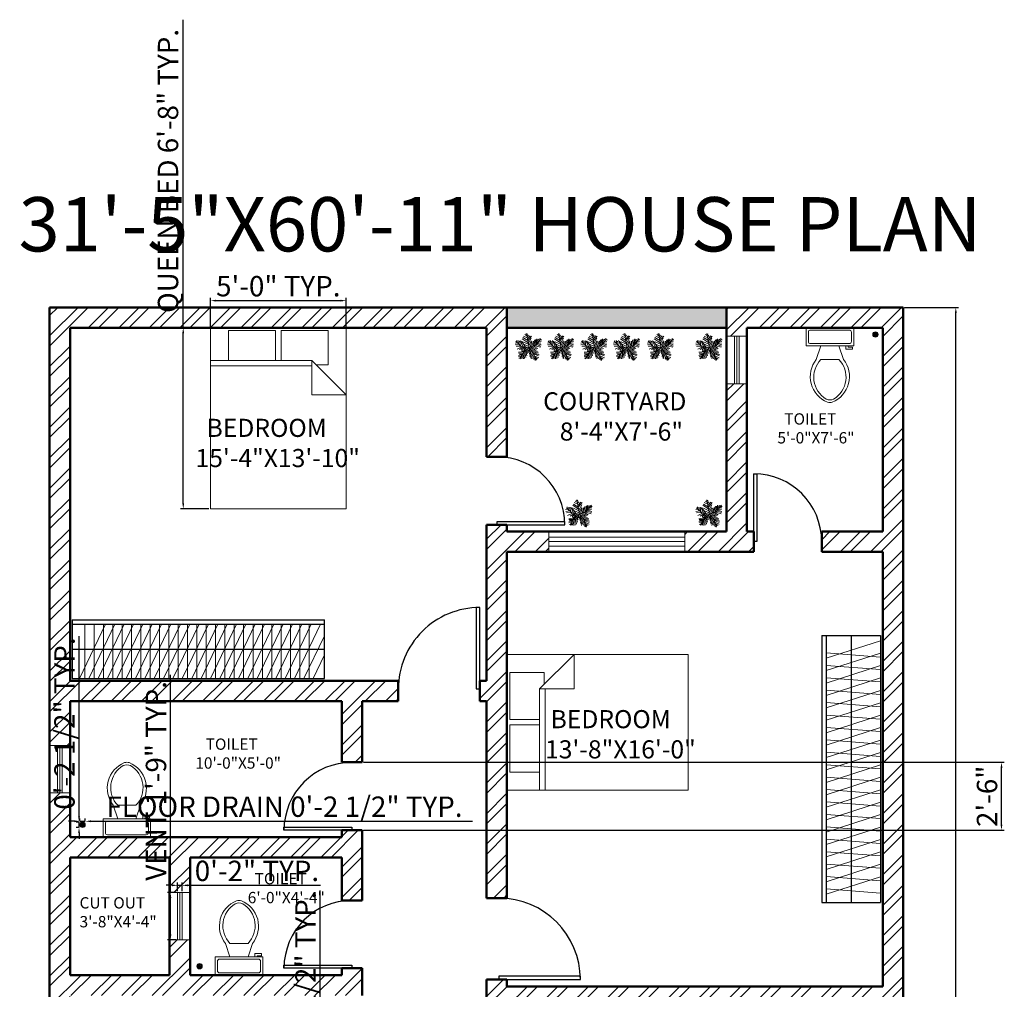
# Model space of a CAD drawing. Units: inches. Extents: x 764 to 1199, y 2696 to 3678.
# Tile 3 of 3: x 764 to 1199, y 3250 to 3678. Entities that reach past the tile are written whole.
import ezdxf

# ---------------------------------------------------------------- set-up
doc = ezdxf.new("R2010")
doc.units = ezdxf.units.IN
for name, color, linetype, lineweight in [('A-ANNO-DIMS', 2, 'Continuous', 18), ('A-ANNO-TITL', 7, 'Continuous', 35), ('A-AREA-IDEN', 7, 'Continuous', 18), ('A-DOOR', 4, 'Continuous', 25), ('A-FLOR-FIXT', 8, 'Continuous', 20), ('A-FURN', 8, 'Continuous', 18), ('A-GLAZ', 244, 'Continuous', 20), ('A-MILL', 8, 'Continuous', 25), ('A-MILL-PATT', 8, 'Continuous', 13), ('A-WALL', 7, 'Continuous', 50), ('A-WALL-PATT', 252, 'Continuous', 13), ('L-PLNT', 3, 'Continuous', 13), ('P-FLOR-DRAN', 8, 'Continuous', 18)]:
    doc.layers.add(name, color=color, linetype=linetype, lineweight=lineweight)
doc.styles.get("Standard").update_dxf_attribs({"font": 'arial.ttf'})
doc.dimstyles.new('ISO-25', dxfattribs={"dimtxt": 9, "dimasz": 2.5, "dimexe": 1.25, "dimexo": 0.625, "dimtad": 1, "dimlunit": 3, "dimtxsty": 'Standard', "dimcen": 2.5, "dimadec": 0, "dimazin": 0, "dimtfac": 1, "dimtmove": 0, "dimatfit": 3, "dimfxl": 1, "dimarcsym": 0})

# ---------------------------------------------------------------- blocks, each defined once
blk = doc.blocks.new('*U2')
for p, q in [((0, 0), (0, -6)), ((40, 0), (40, -6))]:
    blk.add_line(p, q)
blk.add_lwpolyline([(0, 0), (0, 40), (1.75, 40), (1.75, 0)], close=True)
blk.add_arc((0, 0), 40, 0, 90)
blk = doc.blocks.new('*U3')
for p, q in [((0, 0), (0, 6)), ((40, 0), (40, 6))]:
    blk.add_line(p, q)
blk.add_lwpolyline([(0, 0), (0, -40), (1.75, -40), (1.75, 0)], close=True)
blk.add_arc((0, 0), 40, 270, 0)
blk = doc.blocks.new('*U4')
for p, q in [((0, 0), (0, -6)), ((40, 0), (40, -6))]:
    blk.add_line(p, q)
blk.add_lwpolyline([(0, 0), (0, 40), (1.75, 40), (1.75, 0)], close=True)
blk.add_arc((0, 0), 40, 0, 90)
blk = doc.blocks.new('Bed - Queen')
for p, q in [((0, -80.00003), (0, 0)), ((0, 0), (59.99999, 0)), ((59.99999, 0), (59.99999, -80.00003)), ((7.99999, -1.2), (28.79998, -1.2)), ((7.99999, -14.4), (7.99999, -1.2)), ((28.79998, -1.2), (28.79998, -14.4)), ((31.19999, -1.2), (51.99999, -1.2)), ((31.19999, -14.4), (31.19999, -1.2)), ((51.99999, -1.2), (51.99999, -16.4)), ((0, -14.4), (44.8, -14.4)), ((44.8, -16.8), (0, -16.8)), ((59.99999, -29.6), (44.8, -14.4)), ((44.8, -14.4), (44.8, -29.6)), ((51.99999, -16.4), (46.79936, -16.4)), ((44.8, -29.6), (59.99999, -29.6)), ((59.99999, -80.00003), (0, -80.00003))]:
    blk.add_line(p, q)
blk = doc.blocks.new('*U9')
for p, q in [((9.5, -6), (9.5, -2)), ((-10, -8.5), (-8, -8.5)), ((-10, -9.5), (-10, -8.5)), ((-8, -8.5), (-8, -8)), ((-7, -8), (-7, -9.5)), ((-4, -8), (-6, -14)), ((4, -8), (6, -14)), ((-7, -9.5), (-10, -9.5)), ((4, -14), (-4, -14))]:
    blk.add_line(p, q)
blk.add_lwpolyline([(10.5, -8), (10.5, 0), (-10.5, 0), (-10.5, -8)], close=True)
for points in [[(-9.5, -2), (-9.5, -6)], [(8.5, -1), (-8.5, -1)], [(-8.5, -7), (8.5, -7)]]:
    blk.add_lwpolyline(points)
for centre, radius, start, end in [((-8.62, -1.88), 0.884, 81.8699, 188.1301), ((8.62, -1.88), 0.884, 351.8699, 98.1301), ((-8.62, -6.12), 0.884, 171.8699, 278.1301), ((8.62, -6.12), 0.884, 261.8699, 8.1301), ((3.52, -21.58), 12.17, 141.4691, 247.9714), ((4.2, -21.82), 11.33, 136.3677, 238.9468), ((-3.52, -21.58), 12.17, 292.0284, 38.5307), ((-4.2, -21.82), 11.33, 301.053, 43.6321), ((0, -27.88), 4, 245.7318, 294.2682), ((0, -29), 4, 254.8605, 285.1395)]:
    blk.add_arc(centre, radius, start, end)
blk = doc.blocks.new('*U13')
for p, q in [((-5.114, 28.097), (-24.676, 40.636)), ((-7.288, 39.707), (-21.778, 46.673)), ((-8.737, 47.138), (-17.069, 52.711)), ((-10.186, 53.64), (-13.084, 55.962)), ((0, 0), (-10.5, 57)), ((-9.099, 51.782), (-6.563, 55.962)), ((-7.65, 43.423), (-2.578, 49.46)), ((-5.839, 35.992), (4.667, 48.067)), ((-5.114, 27.632), (10.463, 46.673)), ((-47.498, 19.737), (-55.83, 18.344)), ((-40.615, 13.7), (-55.105, 10.913)), ((-31.5, 4.5), (-52.5, 25.5)), ((-33.37, 6.269), (-52.207, 5.34)), ((-48.585, 21.131), (-49.309, 29.026)), ((-28.299, 3.483), (-47.86, -5.805)), ((-43.513, 28.561), (-42.427, 15.558)), ((-38.442, 26.239), (-34.819, 7.663)), ((-21.416, 3.018), (-38.079, -8.128)), ((-35.544, 28.097), (-24.314, 3.947)), ((0, 0), (-31.5, 4.5)), ((-14.533, 2.09), (-30.834, 25.31)), ((-15.982, 2.09), (-30.11, -9.521)), ((-3.665, 19.273), (-27.574, 35.527)), ((-24.314, 23.917), (-2.941, 13.7)), ((0, 0), (-22.5, -19.5)), ((-6.563, 1.161), (-21.416, -8.128)), ((-20.691, 13.7), (-1.129, 4.876)), ((-2.941, 16.486), (8.652, 37.85)), ((-1.129, 6.734), (9.014, 26.704)), ((0, 0), (27, 9)), ((0, 0), (18, -22.5)), ((3.942, 1.625), (11.187, 24.381)), ((6.478, 1.625), (26.04, -8.592)), ((10.101, 3.483), (17.708, 26.239)), ((11.187, 3.483), (30.749, -5.805)), ((16.259, 5.805), (23.142, 31.348)), ((18.07, 5.805), (35.096, -3.483)), ((22.055, 7.198), (27.489, 32.277)), ((24.229, 7.663), (46.688, 1.625)), ((27, 9), (48, 36)), ((27.127, 9.056), (31.112, 35.992)), ((29.662, 12.307), (48.137, 6.269)), ((31.836, 30.883), (32.561, 16.486)), ((33.285, 16.486), (48.862, 10.913)), ((35.096, 32.741), (37.27, 22.524)), ((36.183, 19.737), (48.137, 17.88)), ((38.719, 34.134), (41.979, 28.561)), ((40.53, 25.775), (48.862, 24.846)), ((43.791, 29.954), (51.036, 30.883)), ((44.153, 36.456), (45.239, 32.741)), ((-17.431, -15.094), (-42.789, -18.809)), ((-28.299, -29.026), (-42.789, -31.348)), ((-24.314, -21.596), (-42.427, -22.06)), ((-30.834, -34.135), (-42.427, -35.528)), ((-26.849, -26.24), (-40.253, -25.775)), ((-22.5, -19.5), (-37.5, -45)), ((-32.646, -36.921), (-31.921, -44.352)), ((-15.257, -12.772), (-30.11, -12.772)), ((-29.023, -30.884), (-27.936, -43.887)), ((-25.038, -23.918), (-22.865, -45.281)), ((-20.691, -18.345), (-17.793, -44.352)), ((-6.563, -5.805), (-19.967, -9.985)), ((-17.069, -15.094), (-12.721, -40.172)), ((-13.446, -11.378), (-8.737, -32.741)), ((-9.461, -8.592), (-6.201, -23.453)), ((-4.752, -3.483), (-3.665, -14.629)), ((2.493, -3.019), (-1.491, -20.202)), ((1.769, -2.555), (24.229, -9.521)), ((5.029, -6.27), (2.131, -25.775)), ((9.014, -11.378), (3.58, -35.992)), ((14.085, -16.951), (6.478, -40.172)), ((7.565, -9.056), (32.198, -14.629)), ((18.07, -22.524), (8.289, -45.745)), ((12.274, -15.094), (36.907, -18.809)), ((20.244, -30.419), (15.897, -44.816)), ((16.259, -19.738), (36.183, -22.989)), ((18, -22.5), (27, -52.5)), ((18.433, -22.524), (40.53, -29.026)), ((19.157, -25.311), (38.719, -33.206)), ((22.78, -37.85), (19.519, -48.532)), ((21.331, -32.741), (39.081, -40.636)), ((22.78, -38.314), (34.372, -44.816)), ((-34.457, -39.708), (-40.978, -42.494)), ((24.591, -45.745), (23.142, -50.854)), ((24.591, -43.423), (30.749, -47.603)), ((26.764, -49.925), (28.213, -50.854))]:
    blk.add_line(p, q)
blk = doc.blocks.new('*D15')
at = {"layer": 'A-ANNO-DIMS', "color": 0, "lineweight": -2, "transparency": 16777216}
for p, q in [((1154.86, 3551.25), (1178.72, 3551.25)), ((1177.47, 2822.75), (1177.47, 3548.75)), ((1154.86, 2820.25), (1178.72, 2820.25))]:
    blk.add_line(p, q, dxfattribs=at)
at = {"layer": 'A-ANNO-DIMS', "color": 0, "transparency": 16777216}
for points in [[(1177.05, 3548.75), (1177.89, 3548.75), (1177.47, 3551.25)], [(1177.05, 2822.75), (1177.89, 2822.75), (1177.47, 2820.25)]]:
    blk.add_solid(points, dxfattribs=at)
at = {"layer": 'Defpoints', "color": 0, "transparency": 16777216}
for p in [(1154.24, 3551.25), (1177.47, 3551.25), (1154.24, 2820.25)]:
    blk.add_point(p, dxfattribs=at)
at = {"layer": 'A-ANNO-DIMS', "color": 0, "transparency": 16777216, "insert": (1172.25, 3185.75), "char_height": 9, "attachment_point": 5, "rotation": 90}
blk.add_mtext('60\'-11"', dxfattribs=at)
blk = doc.blocks.new('WIN-GLAZING-60IN')
for p, q in [((0, 4), (60, 4)), ((0, 2), (60, 2)), ((0, 0), (60, 0))]:
    blk.add_line(p, q)
blk = doc.blocks.new('VENT-GLAZING-21IN')
for p, q in [((0, 0), (0, 21)), ((1, 0), (1, 21)), ((2, 0), (2, 21))]:
    blk.add_line(p, q)
blk = doc.blocks.new('FLOOR-DRAIN-ROUND')
for p, q in [((0, 1.19), (2.38, 1.19)), ((2.06, 0.38), (0.32, 2)), ((0.42, 0.28), (1.96, 2.1)), ((1.19, 2.38), (1.19, 0))]:
    blk.add_line(p, q)
for radius in [1.19, 0.891]:
    blk.add_circle((1.19, 1.19), radius)
blk = doc.blocks.new('*D22')
at = {"layer": 'A-ANNO-DIMS', "color": 0, "lineweight": -2, "transparency": 16777216}
for p, q in [((830.59, 3292.75), (830.59, 3388.85)), ((833.11, 3292.75), (829.34, 3292.75)), ((830.59, 3274.25), (830.59, 3290.25)), ((833.11, 3271.75), (829.34, 3271.75))]:
    blk.add_line(p, q, dxfattribs=at)
at = {"layer": 'A-ANNO-DIMS', "color": 0, "transparency": 16777216}
for points in [[(830.17, 3290.25), (831, 3290.25), (830.59, 3292.75)], [(830.17, 3274.25), (831, 3274.25), (830.59, 3271.75)]]:
    blk.add_solid(points, dxfattribs=at)
at = {"layer": 'Defpoints', "color": 0, "transparency": 16777216}
for p in [(830.59, 3292.75), (833.74, 3292.75), (833.74, 3271.75)]:
    blk.add_point(p, dxfattribs=at)
at = {"layer": 'A-ANNO-DIMS', "color": 0, "transparency": 16777216, "insert": (825.37, 3342.05), "char_height": 9, "attachment_point": 5, "rotation": 90}
blk.add_mtext('VENT 1\'-9" TYP.', dxfattribs=at)
blk = doc.blocks.new('*D23')
at = {"layer": 'A-ANNO-DIMS', "color": 0, "lineweight": -2, "transparency": 16777216}
for p, q in [((833.74, 3293.38), (833.74, 3297.15)), ((835.74, 3293.38), (835.74, 3297.15)), ((831.24, 3295.9), (828.74, 3295.9)), ((833.74, 3295.9), (835.74, 3295.9)), ((838.24, 3295.9), (896.85, 3295.9))]:
    blk.add_line(p, q, dxfattribs=at)
at = {"layer": 'A-ANNO-DIMS', "color": 0, "transparency": 16777216}
for points in [[(831.24, 3296.32), (831.24, 3295.48), (833.74, 3295.9)], [(838.24, 3296.32), (838.24, 3295.48), (835.74, 3295.9)]]:
    blk.add_solid(points, dxfattribs=at)
at = {"layer": 'Defpoints', "color": 0, "transparency": 16777216}
for p in [(833.74, 3292.75), (835.74, 3295.9), (835.74, 3292.75)]:
    blk.add_point(p, dxfattribs=at)
at = {"layer": 'A-ANNO-DIMS', "color": 0, "transparency": 16777216, "insert": (868.79, 3301.12), "char_height": 9, "attachment_point": 5}
blk.add_mtext('0\'-2" TYP.', dxfattribs=at)
blk = doc.blocks.new('*D26')
at = {"layer": 'A-ANNO-DIMS', "color": 0, "lineweight": -2, "transparency": 16777216}
for p, q in [((788.08, 3324.2), (785.58, 3324.2)), ((790.58, 3324.47), (790.58, 3325.45)), ((790.58, 3324.2), (792.96, 3324.2)), ((792.96, 3324.47), (792.96, 3325.45)), ((795.46, 3324.2), (963.95, 3324.2))]:
    blk.add_line(p, q, dxfattribs=at)
at = {"layer": 'A-ANNO-DIMS', "color": 0, "transparency": 16777216}
for points in [[(788.08, 3324.62), (788.08, 3323.78), (790.58, 3324.2)], [(795.46, 3324.62), (795.46, 3323.78), (792.96, 3324.2)]]:
    blk.add_solid(points, dxfattribs=at)
at = {"layer": 'Defpoints', "color": 0, "transparency": 16777216}
for p in [(790.58, 3323.84), (792.96, 3324.2), (792.96, 3323.84)]:
    blk.add_point(p, dxfattribs=at)
at = {"layer": 'A-ANNO-DIMS', "color": 0, "transparency": 16777216, "insert": (880.96, 3329.48), "char_height": 9, "attachment_point": 5}
blk.add_mtext('FLOOR DRAIN 0\'-2 1/2" TYP.', dxfattribs=at)
blk = doc.blocks.new('*D27')
at = {"layer": 'A-ANNO-DIMS', "color": 0, "lineweight": -2, "transparency": 16777216}
for p, q in [((790.22, 3326.34), (790.22, 3405.92)), ((789.96, 3323.84), (788.97, 3323.84)), ((790.22, 3321.46), (790.22, 3323.84)), ((789.96, 3321.46), (788.97, 3321.46)), ((790.22, 3318.96), (790.22, 3316.46))]:
    blk.add_line(p, q, dxfattribs=at)
at = {"layer": 'A-ANNO-DIMS', "color": 0, "transparency": 16777216}
for points in [[(789.81, 3326.34), (790.64, 3326.34), (790.22, 3323.84)], [(789.81, 3318.96), (790.64, 3318.96), (790.22, 3321.46)]]:
    blk.add_solid(points, dxfattribs=at)
at = {"layer": 'Defpoints', "color": 0, "transparency": 16777216}
for p in [(790.22, 3323.84), (790.58, 3323.84), (790.58, 3321.46)]:
    blk.add_point(p, dxfattribs=at)
at = {"layer": 'A-ANNO-DIMS', "color": 0, "transparency": 16777216, "insert": (784.94, 3367.38), "char_height": 9, "attachment_point": 5, "rotation": 90}
blk.add_mtext('0\'-2 1/2" TYP.', dxfattribs=at)
blk = doc.blocks.new('*D30')
at = {"layer": 'A-ANNO-DIMS', "color": 0, "lineweight": -2, "transparency": 16777216}
for p, q in [((836.24, 3542.25), (836.24, 3678.39)), ((847.61, 3542.25), (834.99, 3542.25)), ((836.24, 3464.75), (836.24, 3539.75)), ((847.61, 3462.25), (834.99, 3462.25))]:
    blk.add_line(p, q, dxfattribs=at)
at = {"layer": 'A-ANNO-DIMS', "color": 0, "transparency": 16777216}
for points in [[(835.82, 3539.75), (836.65, 3539.75), (836.24, 3542.25)], [(835.82, 3464.75), (836.65, 3464.75), (836.24, 3462.25)]]:
    blk.add_solid(points, dxfattribs=at)
at = {"layer": 'Defpoints', "color": 0, "transparency": 16777216}
for p in [(836.24, 3542.25), (848.24, 3542.25), (848.24, 3462.25)]:
    blk.add_point(p, dxfattribs=at)
at = {"layer": 'A-ANNO-DIMS', "color": 0, "transparency": 16777216, "insert": (830.68, 3611.57), "char_height": 9, "attachment_point": 5, "rotation": 90}
blk.add_mtext('QUEEN BED 6\'-8" TYP.', dxfattribs=at)
blk = doc.blocks.new('*D31')
at = {"layer": 'A-ANNO-DIMS', "color": 0, "lineweight": -2, "transparency": 16777216}
for p, q in [((848.24, 3542.88), (848.24, 3555.5)), ((850.74, 3554.25), (905.74, 3554.25)), ((908.24, 3542.88), (908.24, 3555.5))]:
    blk.add_line(p, q, dxfattribs=at)
at = {"layer": 'A-ANNO-DIMS', "color": 0, "transparency": 16777216}
for points in [[(850.74, 3554.67), (850.74, 3553.83), (848.24, 3554.25)], [(905.74, 3554.67), (905.74, 3553.83), (908.24, 3554.25)]]:
    blk.add_solid(points, dxfattribs=at)
at = {"layer": 'Defpoints', "color": 0, "transparency": 16777216}
for p in [(908.24, 3554.25), (848.24, 3542.25), (908.24, 3542.25)]:
    blk.add_point(p, dxfattribs=at)
at = {"layer": 'A-ANNO-DIMS', "color": 0, "transparency": 16777216, "insert": (878.24, 3559.47), "char_height": 9, "attachment_point": 5}
blk.add_mtext('5\'-0" TYP.', dxfattribs=at)
blk = doc.blocks.new('*D35')
at = {"layer": 'A-ANNO-DIMS', "color": 0, "lineweight": -2, "transparency": 16777216}
for p, q in [((896.66, 3214.06), (896.66, 3293.64)), ((896.66, 3207.94), (896.66, 3211.56)), ((896.74, 3211.56), (897.91, 3211.56)), ((896.66, 3205.44), (896.66, 3202.94)), ((896.74, 3207.94), (897.91, 3207.94))]:
    blk.add_line(p, q, dxfattribs=at)
at = {"layer": 'A-ANNO-DIMS', "color": 0, "transparency": 16777216}
for points in [[(896.24, 3214.06), (897.08, 3214.06), (896.66, 3211.56)], [(896.24, 3205.44), (897.08, 3205.44), (896.66, 3207.94)]]:
    blk.add_solid(points, dxfattribs=at)
at = {"layer": 'Defpoints', "color": 0, "transparency": 16777216}
for p in [(896.12, 3211.56), (896.66, 3211.56), (896.12, 3207.94)]:
    blk.add_point(p, dxfattribs=at)
at = {"layer": 'A-ANNO-DIMS', "color": 0, "transparency": 16777216, "insert": (891.38, 3255.1), "char_height": 9, "attachment_point": 5, "rotation": 90}
blk.add_mtext('0\'-3 1/2" TYP.', dxfattribs=at)
blk = doc.blocks.new('*D37')
at = {"layer": 'A-ANNO-DIMS', "color": 0, "lineweight": -2, "transparency": 16777216}
for p, q in [((915.86, 3350.25), (1198.89, 3350.25)), ((1197.64, 3322.75), (1197.64, 3347.75)), ((915.86, 3320.25), (1198.89, 3320.25))]:
    blk.add_line(p, q, dxfattribs=at)
at = {"layer": 'A-ANNO-DIMS', "color": 0, "transparency": 16777216}
for points in [[(1197.22, 3347.75), (1198.05, 3347.75), (1197.64, 3350.25)], [(1197.22, 3322.75), (1198.05, 3322.75), (1197.64, 3320.25)]]:
    blk.add_solid(points, dxfattribs=at)
at = {"layer": 'Defpoints', "color": 0, "transparency": 16777216}
for p in [(915.24, 3350.25), (1197.64, 3350.25), (915.24, 3320.25)]:
    blk.add_point(p, dxfattribs=at)
at = {"layer": 'A-ANNO-DIMS', "color": 0, "transparency": 16777216, "insert": (1192.42, 3335.25), "char_height": 9, "attachment_point": 5, "rotation": 90}
blk.add_mtext('2\'-6"', dxfattribs=at)

msp = doc.modelspace()

# ---------------------------------------------------------------- hatches: boundary and pattern name
at = {"layer": 'A-MILL-PATT'}
h = msp.add_hatch(dxfattribs=at)
h.set_pattern_fill('ANSI31', color=256, scale=1.172556, angle=19.37869, style=0)
h.paths.add_polyline_path([(787.237, 3387.25), (894.587, 3387.25), (898.716, 3395.86), (898.595, 3404.217), (897.839, 3411.25), (798.747, 3411.25)])
h = msp.add_hatch(dxfattribs=at)
h.set_pattern_fill('ANSI31', color=256, scale=1.300424, angle=45, style=0)
h.paths.add_polyline_path([(791.366, 3387.25), (894.587, 3387.25), (894.587, 3411.25), (791.366, 3411.25)])
h = msp.add_hatch(dxfattribs=at)
h.set_pattern_fill('ANSI31', color=256, scale=1.645192, angle=-27.12835, style=0)
h.paths.add_polyline_path([(1120.237, 3288.25), (1144.237, 3295.989), (1144.237, 3405.756), (1120.237, 3398.017)])
h = msp.add_hatch(dxfattribs=at)
h.set_pattern_fill('ANSI31', color=256, scale=1.723473, angle=130.5845, style=0)
h.paths.add_polyline_path([(1120.237, 3293.739), (1144.237, 3291.886), (1144.237, 3401.652), (1120.237, 3403.505)])
at = {"layer": 'A-WALL-PATT'}
h = msp.add_hatch(dxfattribs=at)
h.set_pattern_fill('ANSI32', color=256)
h.paths.add_polyline_path([(975.237, 2999.25), (960.237, 2999.25), (960.237, 2993.25), (975.237, 2993.25), (975.237, 2966.771), (984.237, 2966.771), (984.237, 3039.25), (987.237, 3039.25), (987.237, 3043.75), (987.237, 3048.25), (984.237, 3048.25), (984.237, 3053.25), (984.237, 3077.25), (975.237, 3077.25), (975.237, 3053.25), (915.237, 3053.25), (906.237, 3053.25), (906.237, 3047.25), (906.237, 2990.25), (910.737, 2990.25), (915.237, 2990.25), (915.237, 2993.25), (930.237, 2993.25), (930.237, 2999.25), (915.237, 2999.25), (915.237, 3047.25), (975.237, 3047.25)])
h.paths.add_polyline_path([(1047.237, 3048.25), (1047.237, 3043.75), (1047.237, 3039.25), (1066.237, 3039.25), (1066.237, 3048.25)])
h.paths.add_polyline_path([(906.237, 2899.25), (876.237, 2899.25), (876.237, 2890.25), (984.237, 2890.25), (984.237, 2945.771), (975.237, 2945.771), (975.237, 2899.25), (915.237, 2899.25), (915.237, 2960.25), (906.237, 2960.25)])
h.paths.add_polyline_path([(786.237, 3047.25), (846.237, 3047.25), (846.237, 3053.25), (786.237, 3053.25), (786.237, 3247.25), (915.237, 3247.25), (915.237, 3259.25), (906.237, 3259.25), (906.237, 3256.25), (839.237, 3256.25), (839.237, 3271.75), (830.237, 3271.75), (830.237, 3256.25), (786.237, 3256.25), (786.237, 3308.25), (830.237, 3308.25), (830.237, 3292.75), (839.237, 3292.75), (839.237, 3308.25), (906.237, 3308.25), (906.237, 3289.25), (915.237, 3289.25), (915.237, 3320.25), (906.237, 3320.25), (906.237, 3317.25), (786.237, 3317.25), (786.237, 3336.75), (777.237, 3336.75), (777.237, 2890.25), (816.237, 2890.25), (816.237, 2899.25), (786.237, 2899.25)])
h.paths.add_polyline_path([(979.237, 3443.25), (997.737, 3443.25), (997.737, 3452.25), (979.237, 3452.25), (979.237, 3455.25), (970.237, 3455.25), (970.237, 3386.25), (967.237, 3386.25), (967.237, 3377.25), (970.237, 3377.25), (970.237, 3290.25), (979.237, 3290.25)])
h.paths.add_polyline_path([(777.237, 3357.75), (786.237, 3357.75), (786.237, 3377.25), (906.237, 3377.25), (906.237, 3350.25), (915.237, 3350.25), (915.237, 3377.25), (931.237, 3377.25), (931.237, 3386.25), (786.237, 3386.25), (786.237, 3542.25), (970.237, 3542.25), (970.237, 3485.25), (979.237, 3485.25), (979.237, 3542.25), (979.237, 3551.25), (777.237, 3551.25)])
h.paths.add_polyline_path([(1076.237, 3452.25), (1057.737, 3452.25), (1057.737, 3443.25), (1076.237, 3443.25), (1088.237, 3443.25), (1088.237, 3452.25), (1085.237, 3452.25), (1085.237, 3517.523), (1076.237, 3517.523)])
h.paths.add_polyline_path([(913.697, 2904.723), (949.086, 2904.723), (949.086, 2931.714), (913.697, 2931.714)], flags=24)
h = msp.add_hatch(color=256, dxfattribs=at)
h.dxf.hatch_style = 1
h.paths.add_polyline_path([(1076.237, 3551.25), (979.237, 3551.25), (979.237, 3542.25), (1076.237, 3542.25)])
h.paths.add_polyline_path([(786.237, 2826.25), (786.237, 2890.25), (777.237, 2890.25), (777.237, 2820.25), (984.237, 2820.25), (984.237, 2826.25)])
h.paths.add_polyline_path([(1154.237, 3039.25), (1145.237, 3039.25), (1145.237, 2826.25), (1136.237, 2826.25), (1136.237, 2820.25), (1154.237, 2820.25)])
h = msp.add_hatch(dxfattribs=at)
h.set_pattern_fill('ANSI32', color=256)
h.paths.add_polyline_path([(1154.237, 3551.25), (1076.237, 3551.25), (1076.237, 3542.25), (1076.237, 3538.523), (1085.237, 3538.523), (1085.237, 3542.25), (1145.237, 3542.25), (1145.237, 3452.25), (1118.237, 3452.25), (1118.237, 3443.25), (1145.237, 3443.25), (1145.237, 3251.25), (979.237, 3251.25), (979.237, 3254.25), (970.237, 3254.25), (970.237, 3242.25), (1145.237, 3242.25), (1145.237, 3048.25), (1126.237, 3048.25), (1126.237, 3039.25), (1154.237, 3039.25)])

# ---------------------------------------------------------------- linework, layer by layer
at = {"layer": 'A-GLAZ'}
for points in [[(1085.237, 3538.523), (1085.237, 3517.523), (1076.237, 3517.523), (1076.237, 3538.523)], [(997.737, 3452.25), (1057.737, 3452.25), (1057.737, 3443.25), (997.737, 3443.25)], [(786.237, 3357.75), (786.237, 3336.75), (777.237, 3336.75), (777.237, 3357.75)], [(839.237, 3292.75), (839.237, 3271.75), (830.237, 3271.75), (830.237, 3292.75)]]:
    msp.add_lwpolyline(points, close=True, dxfattribs=at)
at = {"layer": 'A-MILL'}
for p, q in [((787.237, 3413.25), (787.237, 3387.25)), ((787.237, 3413.25), (898.595, 3413.25)), ((787.237, 3411.25), (898.595, 3411.25)), ((898.595, 3387.25), (898.595, 3413.25)), ((1118.237, 3406.25), (1118.237, 3288.25)), ((1118.237, 3406.25), (1144.237, 3406.25)), ((1120.237, 3406.25), (1120.237, 3288.25)), ((1131.237, 3406.25), (1131.237, 3288.25)), ((1144.237, 3406.25), (1144.237, 3288.25)), ((787.237, 3400.25), (898.595, 3400.25)), ((787.237, 3387.25), (898.595, 3387.25)), ((1118.237, 3288.25), (1144.237, 3288.25))]:
    msp.add_line(p, q, dxfattribs=at)
at = {"layer": 'A-WALL'}
for p, q in [((777.237, 3551.25), (1154.237, 3551.25)), ((777.237, 3551.25), (777.237, 2820.25)), ((979.237, 3542.25), (979.237, 3551.25)), ((1076.237, 3542.25), (1076.237, 3551.25)), ((1154.237, 3551.25), (1154.237, 2820.25)), ((786.237, 3542.25), (970.237, 3542.25)), ((786.237, 3542.25), (786.237, 3386.25)), ((970.237, 3542.25), (970.237, 3485.25)), ((979.237, 3542.25), (1076.237, 3542.25)), ((979.237, 3542.25), (979.237, 3485.25)), ((1076.237, 3542.25), (1076.237, 3452.25)), ((1085.237, 3542.25), (1085.237, 3452.25)), ((1085.237, 3542.25), (1145.237, 3542.25)), ((1145.237, 3542.25), (1145.237, 3452.25)), ((979.237, 3485.25), (970.237, 3485.25)), ((979.237, 3455.25), (970.237, 3455.25)), ((970.237, 3455.25), (970.237, 3386.25)), ((979.237, 3455.25), (979.237, 3452.25)), ((979.237, 3452.25), (1076.237, 3452.25)), ((1085.237, 3452.25), (1088.237, 3452.25)), ((1088.237, 3452.25), (1088.237, 3443.25)), ((1118.237, 3452.25), (1118.237, 3443.25)), ((1118.237, 3452.25), (1145.237, 3452.25)), ((979.237, 3443.25), (1076.237, 3443.25)), ((979.237, 3443.25), (979.237, 3290.25)), ((1076.237, 3443.25), (1088.237, 3443.25)), ((1118.237, 3443.25), (1145.237, 3443.25)), ((1145.237, 3443.25), (1145.237, 3251.25)), ((786.237, 3386.25), (931.237, 3386.25)), ((931.237, 3377.25), (931.237, 3386.25)), ((967.237, 3377.25), (967.237, 3386.25)), ((967.237, 3386.25), (970.237, 3386.25)), ((786.237, 3377.25), (786.237, 3317.25)), ((786.237, 3377.25), (906.237, 3377.25)), ((906.237, 3377.25), (906.237, 3350.25)), ((915.237, 3377.25), (915.237, 3350.25)), ((915.237, 3377.25), (931.237, 3377.25)), ((967.237, 3377.25), (970.237, 3377.25)), ((970.237, 3377.25), (970.237, 3290.25)), ((906.237, 3350.25), (915.237, 3350.25)), ((906.237, 3320.25), (915.237, 3320.25)), ((906.237, 3320.25), (906.237, 3317.25)), ((915.237, 3320.25), (915.237, 3289.25)), ((786.237, 3317.25), (906.237, 3317.25)), ((786.237, 3308.25), (830.237, 3308.25)), ((786.237, 3308.25), (786.237, 3256.25)), ((830.237, 3308.25), (830.237, 3256.25)), ((839.237, 3308.25), (839.237, 3256.25)), ((839.237, 3308.25), (906.237, 3308.25)), ((906.237, 3308.25), (906.237, 3289.25)), ((906.237, 3289.25), (915.237, 3289.25)), ((979.237, 3290.25), (970.237, 3290.25)), ((906.237, 3259.25), (915.237, 3259.25)), ((906.237, 3259.25), (906.237, 3256.25)), ((915.237, 3259.25), (915.237, 3247.25)), ((786.237, 3256.25), (830.237, 3256.25)), ((839.237, 3256.25), (906.237, 3256.25)), ((979.237, 3254.25), (970.237, 3254.25)), ((970.237, 3254.25), (970.237, 3242.25)), ((979.237, 3254.25), (979.237, 3251.25)), ((979.237, 3251.25), (1145.237, 3251.25))]:
    msp.add_line(p, q, dxfattribs=at)

# ---------------------------------------------------------------- block references
at = {"layer": 'A-DOOR'}
for name, p, xscale, yscale, zscale, rotation in [('*U3', (974.737, 3455.25), 0.75, 0.75, 0.75, 90), ('*U3', (967.237, 3382.65), 0.9000000000000136, 0.9000000000000136, 0.9000000000000136, 180), ('*U4', (910.737, 3320.25), 0.75, 0.75, 0.75, 90), ('*U4', (910.737, 3259.25), 0.75, 0.75, 0.75, 90), ('*U3', (975.637, 3254.25), 0.9000000000000136, 0.9000000000000136, 0.9000000000000136, 90)]:
    msp.add_blockref(name, p, dxfattribs=dict(at, xscale=xscale, yscale=yscale, zscale=zscale, rotation=rotation))
at = {"layer": 'A-DOOR', "xscale": 0.75, "yscale": 0.75, "zscale": 0.75}
msp.add_blockref('*U2', (1088.237, 3447.75), dxfattribs=at)
at = {"layer": 'A-FLOR-FIXT', "xscale": -1, "rotation": 359.9999999999971}
msp.add_blockref('*U9', (1121.858, 3542.25), dxfattribs=at)
at = {"layer": 'A-FLOR-FIXT'}
for p, rotation in [((811.344, 3317.25), 180.0000000000029), ((860.867, 3256.25), 180)]:
    msp.add_blockref('*U9', p, dxfattribs=dict(at, rotation=rotation))
at = {"layer": 'A-FURN'}
msp.add_blockref('Bed - Queen', (848.237, 3542.25), dxfattribs=at)
at = {"layer": 'A-FURN', "rotation": 90}
msp.add_blockref('Bed - Queen', (979.237, 3337.95), dxfattribs=at)
at = {"layer": 'A-GLAZ'}
for name, p in [('VENT-GLAZING-21IN', (1079.737, 3517.522)), ('WIN-GLAZING-60IN', (997.737, 3445.75)), ('VENT-GLAZING-21IN', (780.737, 3336.75)), ('VENT-GLAZING-21IN', (833.737, 3271.75))]:
    msp.add_blockref(name, p, dxfattribs=at)
at = {"layer": 'L-PLNT', "xscale": 0.1097639961988601, "yscale": 0.1097639961988601, "zscale": 0.1097639961988601}
for p in [(988.968, 3533.494), (1003.207, 3533.494), (1017.953, 3533.494), (1032.329, 3533.494), (1047.307, 3533.494), (1068.726, 3533.494), (1011.279, 3459.927), (1068.726, 3459.927)]:
    msp.add_blockref('*U13', p, dxfattribs=at)
at = {"layer": 'P-FLOR-DRAN'}
for p in [(1140.787, 3538.089), (790.581, 3321.46), (842.272, 3258.968)]:
    msp.add_blockref('FLOOR-DRAIN-ROUND', p, dxfattribs=at)

# ---------------------------------------------------------------- texts
at = {"layer": 'A-ANNO-TITL', "insert": (763.522, 3599.993), "char_height": 24, "attachment_point": 1}
msp.add_mtext_dynamic_manual_height_columns('31\'-5"X60\'-11" HOUSE PLAN ', width=442.25474, gutter_width=12.5, heights=[0], dxfattribs=at)
at = {"layer": 'A-AREA-IDEN', "attachment_point": 1}
for s, width, insert, char_height in [('COURTYARD\\P   8\'-4"X7\'-6"', 69.80062, (995.2, 3513.75), 8), ('  BEDROOM\\P15\'-4"X13\'-10"', 70.27781, (841.651, 3502.034), 8), ('  TOILET\\P5\'-0"X7\'-6"', 31.84412, (1098.671, 3504.477), 5), (' BEDROOM\\P13\'-8"X16\'-0"', 62.94208, (996.037, 3373.32), 8), ('   TOILET\\P10\'-0"X5\'-0"', 35.68915, (841.58, 3360.778), 5), ('  TOILET\\P6\'-0"X4\'-4"', 35.68915, (864.739, 3301.32), 5), ('CUT OUT\\P3\'-8"X4\'-4"', 35.68915, (790.459, 3290.667), 5)]:
    msp.add_mtext_dynamic_manual_height_columns(s, width=width, gutter_width=12.5, heights=[0], dxfattribs=dict(at, insert=insert, char_height=char_height))

# ---------------------------------------------------------------- dimensions: what is measured, and where the dimension line sits
at = {"layer": 'A-ANNO-DIMS'}
for base, p1, p2, text, picture, middle in [((836.237, 3542.25), (848.237, 3462.25), (848.237, 3542.25), 'QUEEN BED <> TYP.', '*D30', (830.683, 3611.571)), ((790.223, 3323.842), (790.581, 3321.46), (790.581, 3323.842), '<> TYP.', '*D27', (784.945, 3367.383)), ((830.587, 3292.75), (833.737, 3271.75), (833.737, 3292.75), 'VENT <> TYP.', '*D22', (825.367, 3342.051)), ((896.659, 3211.559), (896.117, 3207.942), (896.117, 3211.559), '<> TYP.', '*D35', (891.378, 3255.099))]:
    dim = msp.add_linear_dim(base=base, p1=p1, p2=p2, angle=90, text=text, dimstyle='ISO-25', override={"dimdec": 1, "dimlfac": 1, "dimrnd": 0, "dimzin": 1, "dimdsep": 46, "dimlunit": 4, "dimfrac": 2}, dxfattribs=at)
    dim.commit()
    dim.dimension.update_dxf_attribs({"geometry": picture, "text_midpoint": middle})
for base, p1, p2, text, picture, middle in [((908.237, 3554.25), (848.237, 3542.25), (908.237, 3542.25), '<> TYP.', '*D31', (878.237, 3559.471)), ((792.963, 3324.2), (790.581, 3323.842), (792.963, 3323.842), 'FLOOR DRAIN <> TYP.', '*D26', (880.957, 3329.481)), ((835.737, 3295.9), (833.737, 3292.75), (835.737, 3292.75), '<> TYP.', '*D23', (868.792, 3301.121))]:
    dim = msp.add_linear_dim(base=base, p1=p1, p2=p2, text=text, dimstyle='ISO-25', override={"dimdec": 1, "dimlfac": 1, "dimrnd": 0, "dimzin": 1, "dimdsep": 46, "dimlunit": 4, "dimfrac": 2}, dxfattribs=at)
    dim.commit()
    dim.dimension.update_dxf_attribs({"geometry": picture, "text_midpoint": middle})
for base, p1, p2, override, picture, middle in [((1177.47, 3551.25), (1154.237, 2820.25), (1154.237, 3551.25), {"dimclrd": 0, "dimclre": 0, "dimclrt": 0}, '*D15', (1172.25, 3185.75)), ((1197.637, 3350.25), (915.237, 3320.25), (915.237, 3350.25), {"dimdec": 1, "dimlfac": 1, "dimrnd": 0, "dimzin": 1, "dimdsep": 46, "dimlunit": 4, "dimfrac": 2}, '*D37', (1192.417, 3335.25))]:
    dim = msp.add_linear_dim(base=base, p1=p1, p2=p2, angle=90, dimstyle='ISO-25', override=override, dxfattribs=at)
    dim.commit()
    dim.dimension.update_dxf_attribs({"geometry": picture, "text_midpoint": middle})

doc.saveas('drawing.dxf')
